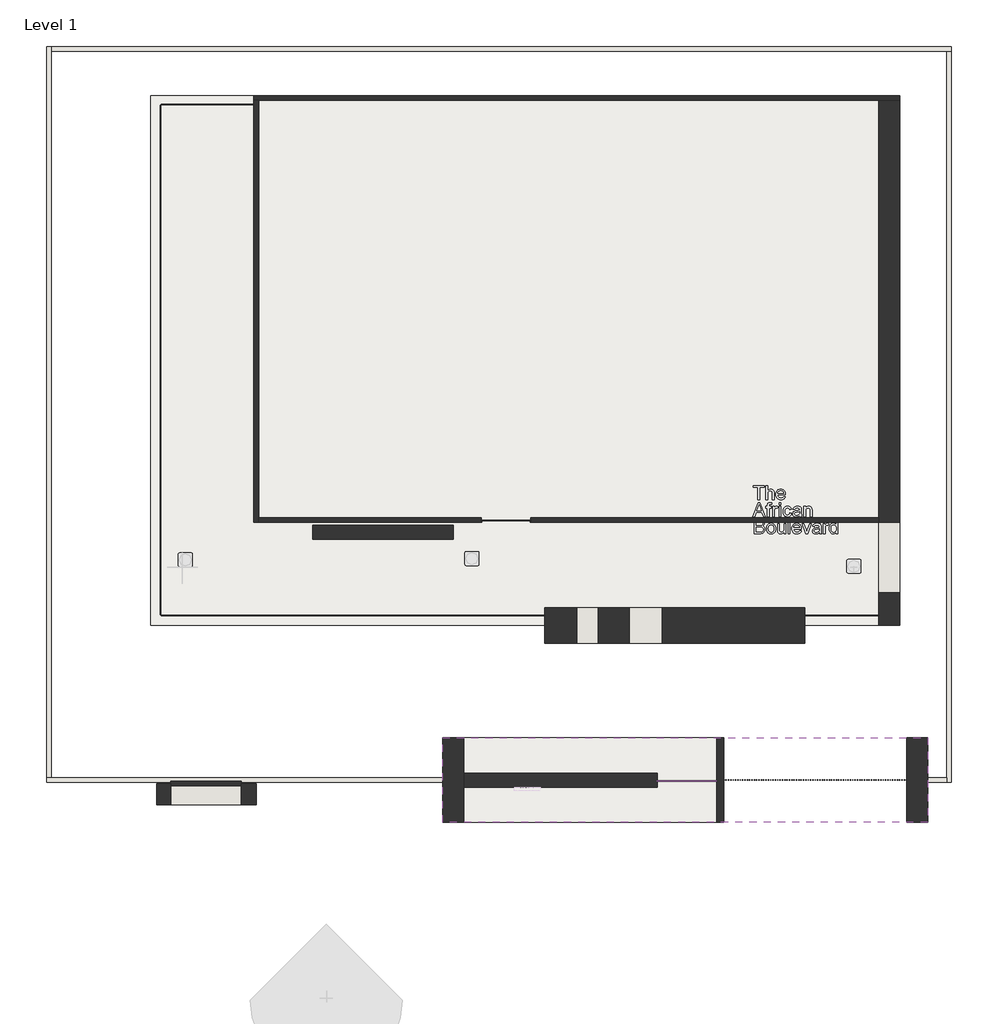
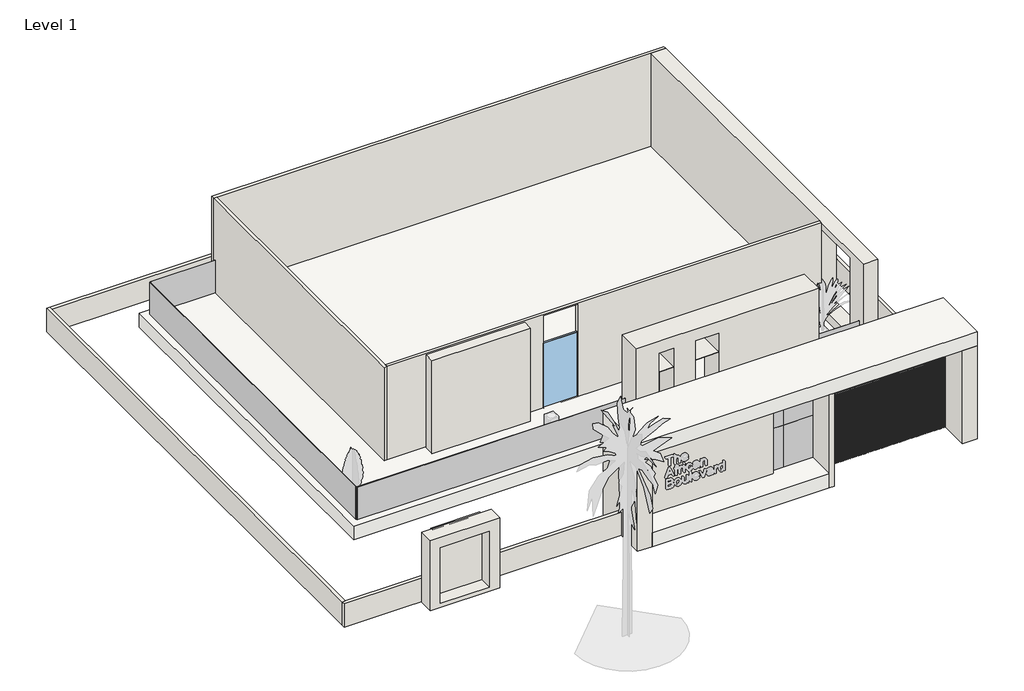
# One storey, part 1 of 3: 17 walls, 8 plates, 3 slabs, 1 railing, 1 window.
"""IFC4 building model written with IfcOpenShell, lengths in millimetres."""

from ifc_helpers import new_model, si_unit, frame, origin, origin_with_axes, place, context, project, spatial, polyline, outline, extrude, faceted_brep, transform, mapped, element, save
from components import system_panel_glazed_7ce5a3c2, system_panel_glazed_6867f845, system_panel_glazed_ba49168f, system_panel_glazed_c41ca4f4, system_panel_glazed_b21aad5f, system_panel_glazed_a143568c, system_panel_glazed_20dba380, system_panel_glazed_7cdb8ab2, window_2382273a

model = new_model("IFC4")

# Units and contexts
model_context = context("Model", 3, world=origin())
ifc_project = project(units=[si_unit("LENGTHUNIT", "METRE", prefix="MILLI")], contexts=[model_context])

# Site, building, storey
site = spatial("IfcSite", under=ifc_project)
building = spatial("IfcBuilding", under=site)
storey = spatial("IfcBuildingStorey", under=building, Name="Level 1", Elevation=0.0)

# Plates
placement = place(None, origin())
system_panel_glazed_shape = system_panel_glazed_7ce5a3c2(model_context)
element("IfcPlate", 1, ObjectType="System Panel : Glazed", at=placement, inside=storey, context=model_context, shape_type="MappedRepresentation", body=[
    mapped(system_panel_glazed_shape, transform((3844.4125281, -5000.7632813, 0.0), x_axis=(-1.0, 0.0, 0.0), y_axis=(0.0, -1.0, 0.0), z_axis=(0.0, 0.0, 1.0))),
])
system_panel_glazed_2_shape = system_panel_glazed_6867f845(model_context)
element("IfcPlate", 2, ObjectType="System Panel : Glazed", at=placement, inside=storey, context=model_context, shape_type="MappedRepresentation", body=[
    mapped(system_panel_glazed_2_shape, transform((-17339.1874719, -5000.7632813, 0.0), x_axis=(-1.0, 0.0, 0.0), y_axis=(0.0, -1.0, 0.0), z_axis=(0.0, 0.0, 1.0))),
])
system_panel_glazed_3_shape = system_panel_glazed_ba49168f(model_context)
element("IfcPlate", 3, ObjectType="System Panel : Glazed", at=placement, inside=storey, context=model_context, shape_type="MappedRepresentation", body=[
    mapped(system_panel_glazed_3_shape, transform((-25644.9874719, 6048.2367187, 0.0), x_axis=(0.0, 1.0, 0.0), y_axis=(-1.0, 0.0, 0.0), z_axis=(0.0, 0.0, 1.0))),
])
system_panel_glazed_4_shape = system_panel_glazed_c41ca4f4(model_context)
element("IfcPlate", 4, ObjectType="System Panel : Glazed", at=placement, inside=storey, context=model_context, shape_type="MappedRepresentation", body=[
    mapped(system_panel_glazed_4_shape, transform((-23638.3874719, 17097.2367187, 0.0), x_axis=(1.0, 0.0, 0.0), y_axis=(0.0, 1.0, 0.0), z_axis=(0.0, 0.0, 1.0))),
])
system_panel_glazed_5_shape = system_panel_glazed_b21aad5f(model_context)
element("IfcPlate", 5, ObjectType="System Panel : Glazed", at=placement, inside=storey, context=model_context, shape_type="MappedRepresentation", body=[
    mapped(system_panel_glazed_5_shape, transform((-2480.1874719, -12163.5632813, -914.4), x_axis=(-1.0, 0.0, 0.0), y_axis=(0.0, -1.0, 0.0), z_axis=(0.0, 0.0, 1.0))),
])
system_panel_glazed_6_shape = system_panel_glazed_a143568c(model_context)
element("IfcPlate", 6, ObjectType="System Panel : Glazed", at=placement, inside=storey, context=model_context, shape_type="MappedRepresentation", body=[
    mapped(system_panel_glazed_6_shape, transform((-2480.1874719, -12163.5632813, 2743.2), x_axis=(-1.0, 0.0, 0.0), y_axis=(0.0, -1.0, 0.0), z_axis=(0.0, 0.0, 1.0))),
])
system_panel_glazed_7_shape = system_panel_glazed_20dba380(model_context)
element("IfcPlate", 7, ObjectType="System Panel : Glazed", at=placement, inside=storey, context=model_context, shape_type="MappedRepresentation", body=[
    mapped(system_panel_glazed_7_shape, transform((-3775.5874719, -12163.5632813, -914.4), x_axis=(-1.0, 0.0, 0.0), y_axis=(0.0, -1.0, 0.0), z_axis=(0.0, 0.0, 1.0))),
])
system_panel_glazed_8_shape = system_panel_glazed_7cdb8ab2(model_context)
element("IfcPlate", 8, ObjectType="System Panel : Glazed", at=placement, inside=storey, context=model_context, shape_type="MappedRepresentation", body=[
    mapped(system_panel_glazed_8_shape, transform((-3775.5874719, -12163.5632813, 2743.2), x_axis=(-1.0, 0.0, 0.0), y_axis=(0.0, -1.0, 0.0), z_axis=(0.0, 0.0, 1.0))),
])

# Railing
element("IfcRailing", 9, ObjectType="Handrail - Rectangular", at=placement, inside=storey, context=model_context, shape_type="SweptSolid", body=[
    extrude(outline(polyline([(6663.8125281, -12138.1632813), (6663.8125281, -12188.9632813), (-1413.3874719, -12188.9632813), (-1413.3874719, -12138.1632813), (6663.8125281, -12138.1632813)])), frame((0.0, 0.0, 3606.8), z_axis=(0.0, 0.0, 1.0), x_axis=(1.0, 0.0, 0.0)), (0.0, 0.0, 1.0), 50.8),
    extrude(outline(polyline([(-1353.0624719, -12154.0382813), (-1353.0624719, -12173.0882813), (-1372.1124719, -12173.0882813), (-1372.1124719, -12154.0382813), (-1353.0624719, -12154.0382813)])), frame((0.0, 0.0, -914.4), z_axis=(0.0, 0.0, 1.0), x_axis=(1.0, 0.0, 0.0)), (0.0, 0.0, 1.0), 4521.2),
    extrude(outline(polyline([(-1251.4624719, -12154.0382813), (-1251.4624719, -12173.0882813), (-1270.5124719, -12173.0882813), (-1270.5124719, -12154.0382813), (-1251.4624719, -12154.0382813)])), frame((0.0, 0.0, -914.4), z_axis=(0.0, 0.0, 1.0), x_axis=(1.0, 0.0, 0.0)), (0.0, 0.0, 1.0), 4521.2),
    extrude(outline(polyline([(-1149.8624719, -12154.0382813), (-1149.8624719, -12173.0882813), (-1168.9124719, -12173.0882813), (-1168.9124719, -12154.0382813), (-1149.8624719, -12154.0382813)])), frame((0.0, 0.0, -914.4), z_axis=(0.0, 0.0, 1.0), x_axis=(1.0, 0.0, 0.0)), (0.0, 0.0, 1.0), 4521.2),
    extrude(outline(polyline([(-1048.2624719, -12154.0382813), (-1048.2624719, -12173.0882813), (-1067.3124719, -12173.0882813), (-1067.3124719, -12154.0382813), (-1048.2624719, -12154.0382813)])), frame((0.0, 0.0, -914.4), z_axis=(0.0, 0.0, 1.0), x_axis=(1.0, 0.0, 0.0)), (0.0, 0.0, 1.0), 4521.2),
    extrude(outline(polyline([(-946.6624719, -12154.0382813), (-946.6624719, -12173.0882813), (-965.7124719, -12173.0882813), (-965.7124719, -12154.0382813), (-946.6624719, -12154.0382813)])), frame((0.0, 0.0, -914.4), z_axis=(0.0, 0.0, 1.0), x_axis=(1.0, 0.0, 0.0)), (0.0, 0.0, 1.0), 4521.2),
    extrude(outline(polyline([(-845.0624719, -12154.0382813), (-845.0624719, -12173.0882813), (-864.1124719, -12173.0882813), (-864.1124719, -12154.0382813), (-845.0624719, -12154.0382813)])), frame((0.0, 0.0, -914.4), z_axis=(0.0, 0.0, 1.0), x_axis=(1.0, 0.0, 0.0)), (0.0, 0.0, 1.0), 4521.2),
    extrude(outline(polyline([(-743.4624719, -12154.0382813), (-743.4624719, -12173.0882813), (-762.5124719, -12173.0882813), (-762.5124719, -12154.0382813), (-743.4624719, -12154.0382813)])), frame((0.0, 0.0, -914.4), z_axis=(0.0, 0.0, 1.0), x_axis=(1.0, 0.0, 0.0)), (0.0, 0.0, 1.0), 4521.2),
    extrude(outline(polyline([(-641.8624719, -12154.0382813), (-641.8624719, -12173.0882813), (-660.9124719, -12173.0882813), (-660.9124719, -12154.0382813), (-641.8624719, -12154.0382813)])), frame((0.0, 0.0, -914.4), z_axis=(0.0, 0.0, 1.0), x_axis=(1.0, 0.0, 0.0)), (0.0, 0.0, 1.0), 4521.2),
    extrude(outline(polyline([(-540.2624719, -12154.0382813), (-540.2624719, -12173.0882813), (-559.3124719, -12173.0882813), (-559.3124719, -12154.0382813), (-540.2624719, -12154.0382813)])), frame((0.0, 0.0, -914.4), z_axis=(0.0, 0.0, 1.0), x_axis=(1.0, 0.0, 0.0)), (0.0, 0.0, 1.0), 4521.2),
    extrude(outline(polyline([(-438.6624719, -12154.0382813), (-438.6624719, -12173.0882813), (-457.7124719, -12173.0882813), (-457.7124719, -12154.0382813), (-438.6624719, -12154.0382813)])), frame((0.0, 0.0, -914.4), z_axis=(0.0, 0.0, 1.0), x_axis=(1.0, 0.0, 0.0)), (0.0, 0.0, 1.0), 4521.2),
    extrude(outline(polyline([(-337.0624719, -12154.0382813), (-337.0624719, -12173.0882813), (-356.1124719, -12173.0882813), (-356.1124719, -12154.0382813), (-337.0624719, -12154.0382813)])), frame((0.0, 0.0, -914.4), z_axis=(0.0, 0.0, 1.0), x_axis=(1.0, 0.0, 0.0)), (0.0, 0.0, 1.0), 4521.2),
    extrude(outline(polyline([(-235.4624719, -12154.0382813), (-235.4624719, -12173.0882813), (-254.5124719, -12173.0882813), (-254.5124719, -12154.0382813), (-235.4624719, -12154.0382813)])), frame((0.0, 0.0, -914.4), z_axis=(0.0, 0.0, 1.0), x_axis=(1.0, 0.0, 0.0)), (0.0, 0.0, 1.0), 4521.2),
    extrude(outline(polyline([(-133.8624719, -12154.0382813), (-133.8624719, -12173.0882813), (-152.9124719, -12173.0882813), (-152.9124719, -12154.0382813), (-133.8624719, -12154.0382813)])), frame((0.0, 0.0, -914.4), z_axis=(0.0, 0.0, 1.0), x_axis=(1.0, 0.0, 0.0)), (0.0, 0.0, 1.0), 4521.2),
    extrude(outline(polyline([(-32.2624719, -12154.0382813), (-32.2624719, -12173.0882813), (-51.3124719, -12173.0882813), (-51.3124719, -12154.0382813), (-32.2624719, -12154.0382813)])), frame((0.0, 0.0, -914.4), z_axis=(0.0, 0.0, 1.0), x_axis=(1.0, 0.0, 0.0)), (0.0, 0.0, 1.0), 4521.2),
    extrude(outline(polyline([(69.3375281, -12154.0382813), (69.3375281, -12173.0882813), (50.2875281, -12173.0882813), (50.2875281, -12154.0382813), (69.3375281, -12154.0382813)])), frame((0.0, 0.0, -914.4), z_axis=(0.0, 0.0, 1.0), x_axis=(1.0, 0.0, 0.0)), (0.0, 0.0, 1.0), 4521.2),
    extrude(outline(polyline([(170.9375281, -12154.0382813), (170.9375281, -12173.0882813), (151.8875281, -12173.0882813), (151.8875281, -12154.0382813), (170.9375281, -12154.0382813)])), frame((0.0, 0.0, -914.4), z_axis=(0.0, 0.0, 1.0), x_axis=(1.0, 0.0, 0.0)), (0.0, 0.0, 1.0), 4521.2),
    extrude(outline(polyline([(272.5375281, -12154.0382813), (272.5375281, -12173.0882813), (253.4875281, -12173.0882813), (253.4875281, -12154.0382813), (272.5375281, -12154.0382813)])), frame((0.0, 0.0, -914.4), z_axis=(0.0, 0.0, 1.0), x_axis=(1.0, 0.0, 0.0)), (0.0, 0.0, 1.0), 4521.2),
    extrude(outline(polyline([(374.1375281, -12154.0382813), (374.1375281, -12173.0882813), (355.0875281, -12173.0882813), (355.0875281, -12154.0382813), (374.1375281, -12154.0382813)])), frame((0.0, 0.0, -914.4), z_axis=(0.0, 0.0, 1.0), x_axis=(1.0, 0.0, 0.0)), (0.0, 0.0, 1.0), 4521.2),
    extrude(outline(polyline([(475.7375281, -12154.0382813), (475.7375281, -12173.0882813), (456.6875281, -12173.0882813), (456.6875281, -12154.0382813), (475.7375281, -12154.0382813)])), frame((0.0, 0.0, -914.4), z_axis=(0.0, 0.0, 1.0), x_axis=(1.0, 0.0, 0.0)), (0.0, 0.0, 1.0), 4521.2),
    extrude(outline(polyline([(577.3375281, -12154.0382813), (577.3375281, -12173.0882813), (558.2875281, -12173.0882813), (558.2875281, -12154.0382813), (577.3375281, -12154.0382813)])), frame((0.0, 0.0, -914.4), z_axis=(0.0, 0.0, 1.0), x_axis=(1.0, 0.0, 0.0)), (0.0, 0.0, 1.0), 4521.2),
    extrude(outline(polyline([(678.9375281, -12154.0382813), (678.9375281, -12173.0882813), (659.8875281, -12173.0882813), (659.8875281, -12154.0382813), (678.9375281, -12154.0382813)])), frame((0.0, 0.0, -914.4), z_axis=(0.0, 0.0, 1.0), x_axis=(1.0, 0.0, 0.0)), (0.0, 0.0, 1.0), 4521.2),
    extrude(outline(polyline([(780.5375281, -12154.0382813), (780.5375281, -12173.0882813), (761.4875281, -12173.0882813), (761.4875281, -12154.0382813), (780.5375281, -12154.0382813)])), frame((0.0, 0.0, -914.4), z_axis=(0.0, 0.0, 1.0), x_axis=(1.0, 0.0, 0.0)), (0.0, 0.0, 1.0), 4521.2),
    extrude(outline(polyline([(882.1375281, -12154.0382813), (882.1375281, -12173.0882813), (863.0875281, -12173.0882813), (863.0875281, -12154.0382813), (882.1375281, -12154.0382813)])), frame((0.0, 0.0, -914.4), z_axis=(0.0, 0.0, 1.0), x_axis=(1.0, 0.0, 0.0)), (0.0, 0.0, 1.0), 4521.2),
    extrude(outline(polyline([(983.7375281, -12154.0382813), (983.7375281, -12173.0882813), (964.6875281, -12173.0882813), (964.6875281, -12154.0382813), (983.7375281, -12154.0382813)])), frame((0.0, 0.0, -914.4), z_axis=(0.0, 0.0, 1.0), x_axis=(1.0, 0.0, 0.0)), (0.0, 0.0, 1.0), 4521.2),
    extrude(outline(polyline([(1085.3375281, -12154.0382813), (1085.3375281, -12173.0882813), (1066.2875281, -12173.0882813), (1066.2875281, -12154.0382813), (1085.3375281, -12154.0382813)])), frame((0.0, 0.0, -914.4), z_axis=(0.0, 0.0, 1.0), x_axis=(1.0, 0.0, 0.0)), (0.0, 0.0, 1.0), 4521.2),
    extrude(outline(polyline([(1186.9375281, -12154.0382813), (1186.9375281, -12173.0882813), (1167.8875281, -12173.0882813), (1167.8875281, -12154.0382813), (1186.9375281, -12154.0382813)])), frame((0.0, 0.0, -914.4), z_axis=(0.0, 0.0, 1.0), x_axis=(1.0, 0.0, 0.0)), (0.0, 0.0, 1.0), 4521.2),
    extrude(outline(polyline([(1288.5375281, -12154.0382813), (1288.5375281, -12173.0882813), (1269.4875281, -12173.0882813), (1269.4875281, -12154.0382813), (1288.5375281, -12154.0382813)])), frame((0.0, 0.0, -914.4), z_axis=(0.0, 0.0, 1.0), x_axis=(1.0, 0.0, 0.0)), (0.0, 0.0, 1.0), 4521.2),
    extrude(outline(polyline([(1390.1375281, -12154.0382813), (1390.1375281, -12173.0882813), (1371.0875281, -12173.0882813), (1371.0875281, -12154.0382813), (1390.1375281, -12154.0382813)])), frame((0.0, 0.0, -914.4), z_axis=(0.0, 0.0, 1.0), x_axis=(1.0, 0.0, 0.0)), (0.0, 0.0, 1.0), 4521.2),
    extrude(outline(polyline([(1491.7375281, -12154.0382813), (1491.7375281, -12173.0882813), (1472.6875281, -12173.0882813), (1472.6875281, -12154.0382813), (1491.7375281, -12154.0382813)])), frame((0.0, 0.0, -914.4), z_axis=(0.0, 0.0, 1.0), x_axis=(1.0, 0.0, 0.0)), (0.0, 0.0, 1.0), 4521.2),
    extrude(outline(polyline([(1593.3375281, -12154.0382813), (1593.3375281, -12173.0882813), (1574.2875281, -12173.0882813), (1574.2875281, -12154.0382813), (1593.3375281, -12154.0382813)])), frame((0.0, 0.0, -914.4), z_axis=(0.0, 0.0, 1.0), x_axis=(1.0, 0.0, 0.0)), (0.0, 0.0, 1.0), 4521.2),
    extrude(outline(polyline([(1694.9375281, -12154.0382813), (1694.9375281, -12173.0882813), (1675.8875281, -12173.0882813), (1675.8875281, -12154.0382813), (1694.9375281, -12154.0382813)])), frame((0.0, 0.0, -914.4), z_axis=(0.0, 0.0, 1.0), x_axis=(1.0, 0.0, 0.0)), (0.0, 0.0, 1.0), 4521.2),
    extrude(outline(polyline([(1796.5375281, -12154.0382813), (1796.5375281, -12173.0882813), (1777.4875281, -12173.0882813), (1777.4875281, -12154.0382813), (1796.5375281, -12154.0382813)])), frame((0.0, 0.0, -914.4), z_axis=(0.0, 0.0, 1.0), x_axis=(1.0, 0.0, 0.0)), (0.0, 0.0, 1.0), 4521.2),
    extrude(outline(polyline([(1898.1375281, -12154.0382813), (1898.1375281, -12173.0882813), (1879.0875281, -12173.0882813), (1879.0875281, -12154.0382813), (1898.1375281, -12154.0382813)])), frame((0.0, 0.0, -914.4), z_axis=(0.0, 0.0, 1.0), x_axis=(1.0, 0.0, 0.0)), (0.0, 0.0, 1.0), 4521.2),
    extrude(outline(polyline([(1999.7375281, -12154.0382813), (1999.7375281, -12173.0882813), (1980.6875281, -12173.0882813), (1980.6875281, -12154.0382813), (1999.7375281, -12154.0382813)])), frame((0.0, 0.0, -914.4), z_axis=(0.0, 0.0, 1.0), x_axis=(1.0, 0.0, 0.0)), (0.0, 0.0, 1.0), 4521.2),
    extrude(outline(polyline([(2101.3375281, -12154.0382813), (2101.3375281, -12173.0882813), (2082.2875281, -12173.0882813), (2082.2875281, -12154.0382813), (2101.3375281, -12154.0382813)])), frame((0.0, 0.0, -914.4), z_axis=(0.0, 0.0, 1.0), x_axis=(1.0, 0.0, 0.0)), (0.0, 0.0, 1.0), 4521.2),
    extrude(outline(polyline([(2202.9375281, -12154.0382813), (2202.9375281, -12173.0882813), (2183.8875281, -12173.0882813), (2183.8875281, -12154.0382813), (2202.9375281, -12154.0382813)])), frame((0.0, 0.0, -914.4), z_axis=(0.0, 0.0, 1.0), x_axis=(1.0, 0.0, 0.0)), (0.0, 0.0, 1.0), 4521.2),
    extrude(outline(polyline([(2304.5375281, -12154.0382813), (2304.5375281, -12173.0882813), (2285.4875281, -12173.0882813), (2285.4875281, -12154.0382813), (2304.5375281, -12154.0382813)])), frame((0.0, 0.0, -914.4), z_axis=(0.0, 0.0, 1.0), x_axis=(1.0, 0.0, 0.0)), (0.0, 0.0, 1.0), 4521.2),
    extrude(outline(polyline([(2406.1375281, -12154.0382813), (2406.1375281, -12173.0882813), (2387.0875281, -12173.0882813), (2387.0875281, -12154.0382813), (2406.1375281, -12154.0382813)])), frame((0.0, 0.0, -914.4), z_axis=(0.0, 0.0, 1.0), x_axis=(1.0, 0.0, 0.0)), (0.0, 0.0, 1.0), 4521.2),
    extrude(outline(polyline([(2507.7375281, -12154.0382813), (2507.7375281, -12173.0882813), (2488.6875281, -12173.0882813), (2488.6875281, -12154.0382813), (2507.7375281, -12154.0382813)])), frame((0.0, 0.0, -914.4), z_axis=(0.0, 0.0, 1.0), x_axis=(1.0, 0.0, 0.0)), (0.0, 0.0, 1.0), 4521.2),
    extrude(outline(polyline([(2609.3375281, -12154.0382813), (2609.3375281, -12173.0882813), (2590.2875281, -12173.0882813), (2590.2875281, -12154.0382813), (2609.3375281, -12154.0382813)])), frame((0.0, 0.0, -914.4), z_axis=(0.0, 0.0, 1.0), x_axis=(1.0, 0.0, 0.0)), (0.0, 0.0, 1.0), 4521.2),
    extrude(outline(polyline([(2710.9375281, -12154.0382813), (2710.9375281, -12173.0882813), (2691.8875281, -12173.0882813), (2691.8875281, -12154.0382813), (2710.9375281, -12154.0382813)])), frame((0.0, 0.0, -914.4), z_axis=(0.0, 0.0, 1.0), x_axis=(1.0, 0.0, 0.0)), (0.0, 0.0, 1.0), 4521.2),
    extrude(outline(polyline([(2812.5375281, -12154.0382813), (2812.5375281, -12173.0882813), (2793.4875281, -12173.0882813), (2793.4875281, -12154.0382813), (2812.5375281, -12154.0382813)])), frame((0.0, 0.0, -914.4), z_axis=(0.0, 0.0, 1.0), x_axis=(1.0, 0.0, 0.0)), (0.0, 0.0, 1.0), 4521.2),
    extrude(outline(polyline([(2914.1375281, -12154.0382813), (2914.1375281, -12173.0882813), (2895.0875281, -12173.0882813), (2895.0875281, -12154.0382813), (2914.1375281, -12154.0382813)])), frame((0.0, 0.0, -914.4), z_axis=(0.0, 0.0, 1.0), x_axis=(1.0, 0.0, 0.0)), (0.0, 0.0, 1.0), 4521.2),
    extrude(outline(polyline([(3015.7375281, -12154.0382813), (3015.7375281, -12173.0882813), (2996.6875281, -12173.0882813), (2996.6875281, -12154.0382813), (3015.7375281, -12154.0382813)])), frame((0.0, 0.0, -914.4), z_axis=(0.0, 0.0, 1.0), x_axis=(1.0, 0.0, 0.0)), (0.0, 0.0, 1.0), 4521.2),
    extrude(outline(polyline([(3117.3375281, -12154.0382813), (3117.3375281, -12173.0882813), (3098.2875281, -12173.0882813), (3098.2875281, -12154.0382813), (3117.3375281, -12154.0382813)])), frame((0.0, 0.0, -914.4), z_axis=(0.0, 0.0, 1.0), x_axis=(1.0, 0.0, 0.0)), (0.0, 0.0, 1.0), 4521.2),
    extrude(outline(polyline([(3218.9375281, -12154.0382813), (3218.9375281, -12173.0882813), (3199.8875281, -12173.0882813), (3199.8875281, -12154.0382813), (3218.9375281, -12154.0382813)])), frame((0.0, 0.0, -914.4), z_axis=(0.0, 0.0, 1.0), x_axis=(1.0, 0.0, 0.0)), (0.0, 0.0, 1.0), 4521.2),
    extrude(outline(polyline([(3320.5375281, -12154.0382813), (3320.5375281, -12173.0882813), (3301.4875281, -12173.0882813), (3301.4875281, -12154.0382813), (3320.5375281, -12154.0382813)])), frame((0.0, 0.0, -914.4), z_axis=(0.0, 0.0, 1.0), x_axis=(1.0, 0.0, 0.0)), (0.0, 0.0, 1.0), 4521.2),
    extrude(outline(polyline([(3422.1375281, -12154.0382813), (3422.1375281, -12173.0882813), (3403.0875281, -12173.0882813), (3403.0875281, -12154.0382813), (3422.1375281, -12154.0382813)])), frame((0.0, 0.0, -914.4), z_axis=(0.0, 0.0, 1.0), x_axis=(1.0, 0.0, 0.0)), (0.0, 0.0, 1.0), 4521.2),
    extrude(outline(polyline([(3523.7375281, -12154.0382813), (3523.7375281, -12173.0882813), (3504.6875281, -12173.0882813), (3504.6875281, -12154.0382813), (3523.7375281, -12154.0382813)])), frame((0.0, 0.0, -914.4), z_axis=(0.0, 0.0, 1.0), x_axis=(1.0, 0.0, 0.0)), (0.0, 0.0, 1.0), 4521.2),
    extrude(outline(polyline([(3625.3375281, -12154.0382813), (3625.3375281, -12173.0882813), (3606.2875281, -12173.0882813), (3606.2875281, -12154.0382813), (3625.3375281, -12154.0382813)])), frame((0.0, 0.0, -914.4), z_axis=(0.0, 0.0, 1.0), x_axis=(1.0, 0.0, 0.0)), (0.0, 0.0, 1.0), 4521.2),
    extrude(outline(polyline([(3726.9375281, -12154.0382813), (3726.9375281, -12173.0882813), (3707.8875281, -12173.0882813), (3707.8875281, -12154.0382813), (3726.9375281, -12154.0382813)])), frame((0.0, 0.0, -914.4), z_axis=(0.0, 0.0, 1.0), x_axis=(1.0, 0.0, 0.0)), (0.0, 0.0, 1.0), 4521.2),
    extrude(outline(polyline([(3828.5375281, -12154.0382813), (3828.5375281, -12173.0882813), (3809.4875281, -12173.0882813), (3809.4875281, -12154.0382813), (3828.5375281, -12154.0382813)])), frame((0.0, 0.0, -914.4), z_axis=(0.0, 0.0, 1.0), x_axis=(1.0, 0.0, 0.0)), (0.0, 0.0, 1.0), 4521.2),
    extrude(outline(polyline([(3930.1375281, -12154.0382813), (3930.1375281, -12173.0882813), (3911.0875281, -12173.0882813), (3911.0875281, -12154.0382813), (3930.1375281, -12154.0382813)])), frame((0.0, 0.0, -914.4), z_axis=(0.0, 0.0, 1.0), x_axis=(1.0, 0.0, 0.0)), (0.0, 0.0, 1.0), 4521.2),
    extrude(outline(polyline([(4031.7375281, -12154.0382813), (4031.7375281, -12173.0882813), (4012.6875281, -12173.0882813), (4012.6875281, -12154.0382813), (4031.7375281, -12154.0382813)])), frame((0.0, 0.0, -914.4), z_axis=(0.0, 0.0, 1.0), x_axis=(1.0, 0.0, 0.0)), (0.0, 0.0, 1.0), 4521.2),
    extrude(outline(polyline([(4133.3375281, -12154.0382813), (4133.3375281, -12173.0882813), (4114.2875281, -12173.0882813), (4114.2875281, -12154.0382813), (4133.3375281, -12154.0382813)])), frame((0.0, 0.0, -914.4), z_axis=(0.0, 0.0, 1.0), x_axis=(1.0, 0.0, 0.0)), (0.0, 0.0, 1.0), 4521.2),
    extrude(outline(polyline([(4234.9375281, -12154.0382813), (4234.9375281, -12173.0882813), (4215.8875281, -12173.0882813), (4215.8875281, -12154.0382813), (4234.9375281, -12154.0382813)])), frame((0.0, 0.0, -914.4), z_axis=(0.0, 0.0, 1.0), x_axis=(1.0, 0.0, 0.0)), (0.0, 0.0, 1.0), 4521.2),
    extrude(outline(polyline([(4336.5375281, -12154.0382813), (4336.5375281, -12173.0882813), (4317.4875281, -12173.0882813), (4317.4875281, -12154.0382813), (4336.5375281, -12154.0382813)])), frame((0.0, 0.0, -914.4), z_axis=(0.0, 0.0, 1.0), x_axis=(1.0, 0.0, 0.0)), (0.0, 0.0, 1.0), 4521.2),
    extrude(outline(polyline([(4438.1375281, -12154.0382813), (4438.1375281, -12173.0882813), (4419.0875281, -12173.0882813), (4419.0875281, -12154.0382813), (4438.1375281, -12154.0382813)])), frame((0.0, 0.0, -914.4), z_axis=(0.0, 0.0, 1.0), x_axis=(1.0, 0.0, 0.0)), (0.0, 0.0, 1.0), 4521.2),
    extrude(outline(polyline([(4539.7375281, -12154.0382813), (4539.7375281, -12173.0882813), (4520.6875281, -12173.0882813), (4520.6875281, -12154.0382813), (4539.7375281, -12154.0382813)])), frame((0.0, 0.0, -914.4), z_axis=(0.0, 0.0, 1.0), x_axis=(1.0, 0.0, 0.0)), (0.0, 0.0, 1.0), 4521.2),
    extrude(outline(polyline([(4641.3375281, -12154.0382813), (4641.3375281, -12173.0882813), (4622.2875281, -12173.0882813), (4622.2875281, -12154.0382813), (4641.3375281, -12154.0382813)])), frame((0.0, 0.0, -914.4), z_axis=(0.0, 0.0, 1.0), x_axis=(1.0, 0.0, 0.0)), (0.0, 0.0, 1.0), 4521.2),
    extrude(outline(polyline([(4742.9375281, -12154.0382813), (4742.9375281, -12173.0882813), (4723.8875281, -12173.0882813), (4723.8875281, -12154.0382813), (4742.9375281, -12154.0382813)])), frame((0.0, 0.0, -914.4), z_axis=(0.0, 0.0, 1.0), x_axis=(1.0, 0.0, 0.0)), (0.0, 0.0, 1.0), 4521.2),
    extrude(outline(polyline([(4844.5375281, -12154.0382813), (4844.5375281, -12173.0882813), (4825.4875281, -12173.0882813), (4825.4875281, -12154.0382813), (4844.5375281, -12154.0382813)])), frame((0.0, 0.0, -914.4), z_axis=(0.0, 0.0, 1.0), x_axis=(1.0, 0.0, 0.0)), (0.0, 0.0, 1.0), 4521.2),
    extrude(outline(polyline([(4946.1375281, -12154.0382813), (4946.1375281, -12173.0882813), (4927.0875281, -12173.0882813), (4927.0875281, -12154.0382813), (4946.1375281, -12154.0382813)])), frame((0.0, 0.0, -914.4), z_axis=(0.0, 0.0, 1.0), x_axis=(1.0, 0.0, 0.0)), (0.0, 0.0, 1.0), 4521.2),
    extrude(outline(polyline([(5047.7375281, -12154.0382813), (5047.7375281, -12173.0882813), (5028.6875281, -12173.0882813), (5028.6875281, -12154.0382813), (5047.7375281, -12154.0382813)])), frame((0.0, 0.0, -914.4), z_axis=(0.0, 0.0, 1.0), x_axis=(1.0, 0.0, 0.0)), (0.0, 0.0, 1.0), 4521.2),
    extrude(outline(polyline([(5149.3375281, -12154.0382813), (5149.3375281, -12173.0882813), (5130.2875281, -12173.0882813), (5130.2875281, -12154.0382813), (5149.3375281, -12154.0382813)])), frame((0.0, 0.0, -914.4), z_axis=(0.0, 0.0, 1.0), x_axis=(1.0, 0.0, 0.0)), (0.0, 0.0, 1.0), 4521.2),
    extrude(outline(polyline([(5250.9375281, -12154.0382813), (5250.9375281, -12173.0882813), (5231.8875281, -12173.0882813), (5231.8875281, -12154.0382813), (5250.9375281, -12154.0382813)])), frame((0.0, 0.0, -914.4), z_axis=(0.0, 0.0, 1.0), x_axis=(1.0, 0.0, 0.0)), (0.0, 0.0, 1.0), 4521.2),
    extrude(outline(polyline([(5352.5375281, -12154.0382813), (5352.5375281, -12173.0882813), (5333.4875281, -12173.0882813), (5333.4875281, -12154.0382813), (5352.5375281, -12154.0382813)])), frame((0.0, 0.0, -914.4), z_axis=(0.0, 0.0, 1.0), x_axis=(1.0, 0.0, 0.0)), (0.0, 0.0, 1.0), 4521.2),
    extrude(outline(polyline([(5454.1375281, -12154.0382813), (5454.1375281, -12173.0882813), (5435.0875281, -12173.0882813), (5435.0875281, -12154.0382813), (5454.1375281, -12154.0382813)])), frame((0.0, 0.0, -914.4), z_axis=(0.0, 0.0, 1.0), x_axis=(1.0, 0.0, 0.0)), (0.0, 0.0, 1.0), 4521.2),
    extrude(outline(polyline([(5555.7375281, -12154.0382813), (5555.7375281, -12173.0882813), (5536.6875281, -12173.0882813), (5536.6875281, -12154.0382813), (5555.7375281, -12154.0382813)])), frame((0.0, 0.0, -914.4), z_axis=(0.0, 0.0, 1.0), x_axis=(1.0, 0.0, 0.0)), (0.0, 0.0, 1.0), 4521.2),
    extrude(outline(polyline([(5657.3375281, -12154.0382813), (5657.3375281, -12173.0882813), (5638.2875281, -12173.0882813), (5638.2875281, -12154.0382813), (5657.3375281, -12154.0382813)])), frame((0.0, 0.0, -914.4), z_axis=(0.0, 0.0, 1.0), x_axis=(1.0, 0.0, 0.0)), (0.0, 0.0, 1.0), 4521.2),
    extrude(outline(polyline([(5758.9375281, -12154.0382813), (5758.9375281, -12173.0882813), (5739.8875281, -12173.0882813), (5739.8875281, -12154.0382813), (5758.9375281, -12154.0382813)])), frame((0.0, 0.0, -914.4), z_axis=(0.0, 0.0, 1.0), x_axis=(1.0, 0.0, 0.0)), (0.0, 0.0, 1.0), 4521.2),
    extrude(outline(polyline([(5860.5375281, -12154.0382813), (5860.5375281, -12173.0882813), (5841.4875281, -12173.0882813), (5841.4875281, -12154.0382813), (5860.5375281, -12154.0382813)])), frame((0.0, 0.0, -914.4), z_axis=(0.0, 0.0, 1.0), x_axis=(1.0, 0.0, 0.0)), (0.0, 0.0, 1.0), 4521.2),
    extrude(outline(polyline([(5962.1375281, -12154.0382813), (5962.1375281, -12173.0882813), (5943.0875281, -12173.0882813), (5943.0875281, -12154.0382813), (5962.1375281, -12154.0382813)])), frame((0.0, 0.0, -914.4), z_axis=(0.0, 0.0, 1.0), x_axis=(1.0, 0.0, 0.0)), (0.0, 0.0, 1.0), 4521.2),
    extrude(outline(polyline([(6063.7375281, -12154.0382813), (6063.7375281, -12173.0882813), (6044.6875281, -12173.0882813), (6044.6875281, -12154.0382813), (6063.7375281, -12154.0382813)])), frame((0.0, 0.0, -914.4), z_axis=(0.0, 0.0, 1.0), x_axis=(1.0, 0.0, 0.0)), (0.0, 0.0, 1.0), 4521.2),
    extrude(outline(polyline([(6165.3375281, -12154.0382813), (6165.3375281, -12173.0882813), (6146.2875281, -12173.0882813), (6146.2875281, -12154.0382813), (6165.3375281, -12154.0382813)])), frame((0.0, 0.0, -914.4), z_axis=(0.0, 0.0, 1.0), x_axis=(1.0, 0.0, 0.0)), (0.0, 0.0, 1.0), 4521.2),
    extrude(outline(polyline([(6266.9375281, -12154.0382813), (6266.9375281, -12173.0882813), (6247.8875281, -12173.0882813), (6247.8875281, -12154.0382813), (6266.9375281, -12154.0382813)])), frame((0.0, 0.0, -914.4), z_axis=(0.0, 0.0, 1.0), x_axis=(1.0, 0.0, 0.0)), (0.0, 0.0, 1.0), 4521.2),
    extrude(outline(polyline([(6368.5375281, -12154.0382813), (6368.5375281, -12173.0882813), (6349.4875281, -12173.0882813), (6349.4875281, -12154.0382813), (6368.5375281, -12154.0382813)])), frame((0.0, 0.0, -914.4), z_axis=(0.0, 0.0, 1.0), x_axis=(1.0, 0.0, 0.0)), (0.0, 0.0, 1.0), 4521.2),
    extrude(outline(polyline([(6470.1375281, -12154.0382813), (6470.1375281, -12173.0882813), (6451.0875281, -12173.0882813), (6451.0875281, -12154.0382813), (6470.1375281, -12154.0382813)])), frame((0.0, 0.0, -914.4), z_axis=(0.0, 0.0, 1.0), x_axis=(1.0, 0.0, 0.0)), (0.0, 0.0, 1.0), 4521.2),
    extrude(outline(polyline([(6571.7375281, -12154.0382813), (6571.7375281, -12173.0882813), (6552.6875281, -12173.0882813), (6552.6875281, -12154.0382813), (6571.7375281, -12154.0382813)])), frame((0.0, 0.0, -914.4), z_axis=(0.0, 0.0, 1.0), x_axis=(1.0, 0.0, 0.0)), (0.0, 0.0, 1.0), 4521.2),
    extrude(outline(polyline([(-1394.3374719, -12154.0382813), (-1394.3374719, -12173.0882813), (-1413.3874719, -12173.0882813), (-1413.3874719, -12154.0382813), (-1394.3374719, -12154.0382813)])), frame((0.0, 0.0, -914.4), z_axis=(0.0, 0.0, 1.0), x_axis=(1.0, 0.0, 0.0)), (0.0, 0.0, 1.0), 4521.2),
    extrude(outline(polyline([(6663.8125281, -12154.0382813), (6663.8125281, -12173.0882813), (6644.7625281, -12173.0882813), (6644.7625281, -12154.0382813), (6663.8125281, -12154.0382813)])), frame((0.0, 0.0, -914.4), z_axis=(0.0, 0.0, 1.0), x_axis=(1.0, 0.0, 0.0)), (0.0, 0.0, 1.0), 4521.2),
])

# Slabs
element("IfcSlab", 10, ObjectType="Generic - 3'", at=placement, inside=storey, context=model_context, shape_type="SweptSolid", body=[
    extrude(outline(polyline([(-26102.1874719, -5457.9632813), (-26102.1874719, 17503.6367187), (6359.0125281, 17503.6367187), (6359.0125281, -5457.9632813), (-26102.1874719, -5457.9632813)])), frame((0.0, 0.0, -914.4), z_axis=(0.0, 0.0, 1.0), x_axis=(1.0, 0.0, 0.0)), (0.0, 0.0, 1.0), 914.4),
])
element("IfcSlab", 11, ObjectType="Generic - 3'", at=placement, inside=storey, context=model_context, shape_type="SweptSolid", body=[
    extrude(outline(polyline([(-1565.7874719, -10334.7632813), (-1565.7874719, -13992.3632813), (-12538.5874719, -13992.3632813), (-12538.5874719, -10334.7632813), (-1565.7874719, -10334.7632813)])), frame((0.0, 0.0, -914.4), z_axis=(0.0, 0.0, 1.0), x_axis=(1.0, 0.0, 0.0)), (0.0, 0.0, 1.0), 914.4),
])
element("IfcSlab", 12, ObjectType="Generic - 3'", at=placement, inside=storey, context=model_context, shape_type="SweptSolid", body=[
    extrude(outline(polyline([(7578.2125281, -10334.7632813), (7578.2125281, -13992.3632813), (-13452.9874719, -13992.3632813), (-13452.9874719, -10334.7632813), (7578.2125281, -10334.7632813)])), frame((0.0, 0.0, 5181.6), z_axis=(0.0, 0.0, 1.0), x_axis=(1.0, 0.0, 0.0)), (0.0, 0.0, 1.0), 914.4),
])

# Walls
element("IfcWall", 13, ObjectType="Generic - 12\" 2", at=placement, inside=storey, context=model_context, shape_type="SweptSolid", body=[
    extrude(outline(polyline([(-1565.7874719, -13992.3632813), (-1565.7874719, -10334.7632813), (-1260.9874719, -10334.7632813), (-1260.9874719, -13992.3632813), (-1565.7874719, -13992.3632813)])), frame((0.0, 0.0, -914.4), z_axis=(0.0, 0.0, 1.0), x_axis=(1.0, 0.0, 0.0)), (0.0, 0.0, 1.0), 6096.0),
])
element("IfcWall", 14, ObjectType="Generic - 3'", at=placement, inside=storey, context=model_context, shape_type="Brep", body=[
    faceted_brep([(5444.6125281, 17300.4367187, 0.0), (5444.6125281, -784.3632813, 0.0), (5444.6125281, -987.5632813, 0.0), (5444.6125281, -5457.9632813, 0.0), (5444.6125281, -5457.9632813, 6096.0), (5444.6125281, -987.5632813, 6096.0), (5444.6125281, -784.3632813, 6096.0), (5444.6125281, 17300.4367187, 6096.0), (5444.6125281, -4035.5632813, 5648.487938), (5444.6125281, -4035.5632813, 619.287938), (5444.6125281, -987.5632813, 619.287938), (5444.6125281, -987.5632813, 5648.487938), (6359.0125281, 17300.4367187, 0.0), (6359.0125281, 17300.4367187, 6096.0), (6359.0125281, -5457.9632813, 6096.0), (6359.0125281, -5457.9632813, 0.0), (6359.0125281, -4035.5632813, 5648.487938), (6359.0125281, -987.5632813, 5648.487938), (6359.0125281, -987.5632813, 619.287938), (6359.0125281, -4035.5632813, 619.287938)], [[[0, 1, 2, 3, 4, 5, 6, 7], [8, 9, 10, 11]], [[12, 13, 14, 15], [16, 17, 18, 19]], [[0, 7, 13, 12]], [[3, 2, 1, 0, 12, 15]], [[4, 3, 15, 14]], [[7, 6, 5, 4, 14, 13]], [[9, 8, 16, 19]], [[10, 9, 19, 18]], [[8, 11, 17, 16]], [[11, 10, 18, 17]]]),
])
element("IfcWall", 15, ObjectType="Generic - 3'", at=placement, inside=storey, context=model_context, shape_type="Brep", body=[
    faceted_brep([(-13452.9874719, -10334.7632813, -914.4), (-13452.9874719, -12061.9632813, -914.4), (-13452.9874719, -12265.1632813, -914.4), (-13452.9874719, -13992.3632813, -914.4), (-13452.9874719, -13992.3632813, 5181.6), (-13452.9874719, -10334.7632813, 5181.6), (-12538.5874719, -10334.7632813, -914.4), (-12538.5874719, -10334.7632813, 5181.6), (-12538.5874719, -11858.7632813, 5181.6), (-12538.5874719, -12468.3632813, 5181.6), (-12538.5874719, -13992.3632813, 5181.6), (-12538.5874719, -13992.3632813, -914.4), (-12538.5874719, -12468.3632813, -914.4), (-12538.5874719, -11858.7632813, -914.4)], [[[0, 1, 2, 3, 4, 5]], [[6, 7, 8, 9, 10, 11, 12, 13]], [[3, 2, 1, 0, 6, 13, 12, 11]], [[4, 3, 11, 10]], [[5, 4, 10, 9, 8, 7]], [[0, 5, 7, 6]]]),
])
element("IfcWall", 16, ObjectType="Generic - 3'", at=placement, inside=storey, context=model_context, shape_type="Brep", body=[
    faceted_brep([(6663.8125281, -10334.7632813, -914.4), (6663.8125281, -13992.3632813, -914.4), (6663.8125281, -13992.3632813, 5181.6), (6663.8125281, -10334.7632813, 5181.6), (7578.2125281, -10334.7632813, -914.4), (7578.2125281, -10334.7632813, 5181.6), (7578.2125281, -13992.3632813, 5181.6), (7578.2125281, -13992.3632813, -914.4), (7578.2125281, -12265.1632813, -914.4), (7578.2125281, -12061.9632813, -914.4)], [[[0, 1, 2, 3]], [[4, 5, 6, 7, 8, 9]], [[1, 0, 4, 9, 8, 7]], [[2, 1, 7, 6]], [[3, 2, 6, 5]], [[0, 3, 5, 4]]]),
])
element("IfcWall", 17, ObjectType="Generic - 3'", at=placement, inside=storey, context=model_context, shape_type="SweptSolid", body=[
    extrude(outline(polyline([(-914.4, -25838.6624719), (-914.4, -21530.1874719), (3657.6, -21530.1874719), (3657.6, -25838.6624719), (-914.4, -25838.6624719)]), holes=[polyline([(2997.2, -22181.0624719), (-660.4, -22181.0624719), (-660.4, -25229.0624719), (2997.2, -25229.0624719), (2997.2, -22181.0624719)])]), frame((0.0, -13230.3632813, 0.0), z_axis=(0.0, 1.0, 0.0), x_axis=(0.0, 0.0, 1.0)), (0.0, 0.0, 1.0), 914.4),
])
element("IfcWall", 18, ObjectType="Generic - 3' gray", at=placement, inside=storey, context=model_context, shape_type="SweptSolid", body=[
    extrude(outline(polyline([(0.0, 2244.2125281), (6096.0, 2244.2125281), (6096.0, -9033.3874719), (0.0, -9033.3874719), (0.0, 2244.2125281)]), holes=[polyline([(5315.3308744, -6716.0306948), (4096.1308744, -6716.0306948), (4096.1308744, -7630.4306948), (5315.3308744, -7630.4306948), (5315.3308744, -6716.0306948)]), polyline([(286.1308744, -7630.4306948), (4070.7308744, -7630.4306948), (4070.7308744, -6716.0306948), (286.1308744, -6716.0306948), (286.1308744, -7630.4306948)]), polyline([(5315.3308744, -3924.8577662), (4096.1308744, -3924.8577662), (4096.1308744, -5371.4183212), (5315.3308744, -5371.4183212), (5315.3308744, -3924.8577662)]), polyline([(286.1308744, -5371.4183212), (4070.7308744, -5371.4183212), (4070.7308744, -3924.8577662), (286.1308744, -3924.8577662), (286.1308744, -5371.4183212)])]), frame((0.0, -6219.9632813, 0.0), z_axis=(0.0, 1.0, 0.0), x_axis=(0.0, 0.0, 1.0)), (0.0, 0.0, 1.0), 1524.0),
])
element("IfcWall", 19, ObjectType="Generic - 8\"", at=placement, inside=storey, context=model_context, shape_type="Brep", body=[
    faceted_brep([(-21631.7874719, 17300.4367187, 0.0), (-21428.5874719, 17300.4367187, 0.0), (5444.6125281, 17300.4367187, 0.0), (6359.0125281, 17300.4367187, 0.0), (6359.0125281, 17300.4367187, 6096.0), (5444.6125281, 17300.4367187, 6096.0), (-21428.5874719, 17300.4367187, 6096.0), (-21631.7874719, 17300.4367187, 6096.0), (-21631.7874719, 17503.6367187, 0.0), (-21631.7874719, 17503.6367187, 6096.0), (6359.0125281, 17503.6367187, 6096.0), (6359.0125281, 17503.6367187, 0.0)], [[[0, 1, 2, 3, 4, 5, 6, 7]], [[8, 9, 10, 11]], [[3, 2, 1, 0, 8, 11]], [[7, 6, 5, 4, 10, 9]], [[0, 7, 9, 8]], [[4, 3, 11, 10]]]),
])
element("IfcWall", 20, ObjectType="Generic - 8\"", at=placement, inside=storey, context=model_context, shape_type="Brep", body=[
    faceted_brep([(-21428.5874719, -987.5632813, 0.0), (-21428.5874719, -784.3632813, 0.0), (-21428.5874719, 17300.4367187, 0.0), (-21428.5874719, 17300.4367187, 6096.0), (-21428.5874719, -784.3632813, 6096.0), (-21428.5874719, -987.5632813, 6096.0), (-21631.7874719, -987.5632813, 0.0), (-21631.7874719, -987.5632813, 6096.0), (-21631.7874719, 17300.4367187, 6096.0), (-21631.7874719, 17300.4367187, 0.0)], [[[0, 1, 2, 3, 4, 5]], [[6, 7, 8, 9]], [[2, 1, 0, 6, 9]], [[5, 4, 3, 8, 7]], [[0, 5, 7, 6]], [[3, 2, 9, 8]]]),
])
element("IfcWall", 21, ObjectType="Generic - 8\"", at=placement, inside=storey, context=model_context, shape_type="Brep", body=[
    faceted_brep([(-21428.5874719, -784.3632813, 6096.0), (5444.6125281, -784.3632813, 6096.0), (5444.6125281, -784.3632813, 0.0), (-9642.9874719, -784.3632813, 0.0), (-9642.9874719, -784.3632813, 6034.6483945), (-11776.5874719, -784.3632813, 6034.6483945), (-11776.5874719, -784.3632813, 0.0), (-21428.5874719, -784.3632813, 0.0), (5444.6125281, -987.5632813, 6096.0), (-21428.5874719, -987.5632813, 6096.0), (-21428.5874719, -987.5632813, 0.0), (-11776.5874719, -987.5632813, 0.0), (-11776.5874719, -987.5632813, 6034.6483945), (-9642.9874719, -987.5632813, 6034.6483945), (-9642.9874719, -987.5632813, 0.0), (5444.6125281, -987.5632813, 0.0), (5444.6125281, -987.5632813, 619.287938), (5444.6125281, -987.5632813, 5648.487938)], [[[0, 1, 2, 3, 4, 5, 6, 7]], [[8, 9, 10, 11, 12, 13, 14, 15, 16, 17]], [[10, 7, 6, 11]], [[3, 2, 15, 14]], [[1, 0, 9, 8]], [[0, 7, 10, 9]], [[11, 6, 5, 12]], [[3, 14, 13, 4]], [[12, 5, 4, 13]], [[15, 2, 1, 8, 17, 16]]]),
])
element("IfcWall", 22, ObjectType="Generic - 8\" 2", at=placement, inside=storey, context=model_context, shape_type="Brep", body=[
    faceted_brep([(-13452.9874719, -12061.9632813, -914.4), (-30420.1874719, -12061.9632813, -914.4), (-30623.3874719, -12061.9632813, -914.4), (-30623.3874719, -12061.9632813, 609.6), (-30420.1874719, -12061.9632813, 609.6), (-13452.9874719, -12061.9632813, 609.6), (-13452.9874719, -12265.1632813, -914.4), (-13452.9874719, -12265.1632813, 609.6), (-30623.3874719, -12265.1632813, 609.6), (-30623.3874719, -12265.1632813, -914.4)], [[[0, 1, 2, 3, 4, 5]], [[6, 7, 8, 9]], [[2, 1, 0, 6, 9]], [[5, 4, 3, 8, 7]], [[0, 5, 7, 6]], [[3, 2, 9, 8]]]),
])
element("IfcWall", 23, ObjectType="Generic - 8\" 2", at=placement, inside=storey, context=model_context, shape_type="Brep", body=[
    faceted_brep([(-30420.1874719, -12061.9632813, -914.4), (-30420.1874719, 19434.0367187, -914.4), (-30420.1874719, 19637.2367187, -914.4), (-30420.1874719, 19637.2367187, 609.6), (-30420.1874719, 19434.0367187, 609.6), (-30420.1874719, -12061.9632813, 609.6), (-30623.3874719, -12061.9632813, -914.4), (-30623.3874719, -12061.9632813, 609.6), (-30623.3874719, 19637.2367187, 609.6), (-30623.3874719, 19637.2367187, -914.4)], [[[0, 1, 2, 3, 4, 5]], [[6, 7, 8, 9]], [[2, 1, 0, 6, 9]], [[5, 4, 3, 8, 7]], [[0, 5, 7, 6]], [[3, 2, 9, 8]]]),
])
element("IfcWall", 24, ObjectType="Generic - 8\" 2", at=placement, inside=storey, context=model_context, shape_type="Brep", body=[
    faceted_brep([(-30420.1874719, 19434.0367187, -914.4), (8391.0125281, 19434.0367187, -914.4), (8594.2125281, 19434.0367187, -914.4), (8594.2125281, 19434.0367187, 609.6), (8391.0125281, 19434.0367187, 609.6), (-30420.1874719, 19434.0367187, 609.6), (-30420.1874719, 19637.2367187, -914.4), (-30420.1874719, 19637.2367187, 609.6), (8594.2125281, 19637.2367187, 609.6), (8594.2125281, 19637.2367187, -914.4)], [[[0, 1, 2, 3, 4, 5]], [[6, 7, 8, 9]], [[2, 1, 0, 6, 9]], [[5, 4, 3, 8, 7]], [[0, 5, 7, 6]], [[3, 2, 9, 8]]]),
])
element("IfcWall", 25, ObjectType="Generic - 8\" 2", at=placement, inside=storey, context=model_context, shape_type="Brep", body=[
    faceted_brep([(8391.0125281, 19434.0367187, -914.4), (8391.0125281, -12061.9632813, -914.4), (8391.0125281, -12265.1632813, -914.4), (8391.0125281, -12265.1632813, 609.6), (8391.0125281, -12061.9632813, 609.6), (8391.0125281, 19434.0367187, 609.6), (8594.2125281, 19434.0367187, -914.4), (8594.2125281, 19434.0367187, 609.6), (8594.2125281, -12265.1632813, 609.6), (8594.2125281, -12265.1632813, -914.4)], [[[0, 1, 2, 3, 4, 5]], [[6, 7, 8, 9]], [[2, 1, 0, 6, 9]], [[5, 4, 3, 8, 7]], [[0, 5, 7, 6]], [[3, 2, 9, 8]]]),
])
element("IfcWall", 26, ObjectType="Generic - 8\" 2", at=placement, inside=storey, context=model_context, shape_type="SweptSolid", body=[
    extrude(outline(polyline([(8391.0125281, -12265.1632813), (7578.2125281, -12265.1632813), (7578.2125281, -12061.9632813), (8391.0125281, -12061.9632813), (8391.0125281, -12265.1632813)])), frame((0.0, 0.0, -914.4), z_axis=(0.0, 0.0, 1.0), x_axis=(1.0, 0.0, 0.0)), (0.0, 0.0, 1.0), 1524.0),
])
element("IfcWall", 27, ObjectType="Generic - 8\" 2", at=placement, inside=storey, context=model_context, shape_type="SweptSolid", body=[
    extrude(outline(polyline([(-22181.0624719, -12417.5632813), (-25229.0624719, -12417.5632813), (-25229.0624719, -12214.3632813), (-22181.0624719, -12214.3632813), (-22181.0624719, -12417.5632813)])), frame((0.0, 0.0, -914.4), z_axis=(0.0, 0.0, 1.0), x_axis=(1.0, 0.0, 0.0)), (0.0, 0.0, 1.0), 4572.0),
])
element("IfcWall", 28, ObjectType="Generic -2", at=placement, inside=storey, context=model_context, shape_type="SweptSolid", body=[
    extrude(outline(polyline([(-12995.7874719, -1724.1632813), (-19091.7874719, -1724.1632813), (-19091.7874719, -1114.5632813), (-12995.7874719, -1114.5632813), (-12995.7874719, -1724.1632813)])), origin_with_axes(), (0.0, 0.0, 1.0), 6106.1211964),
])
element("IfcWall", 29, ObjectType="Generic -2", at=placement, inside=storey, context=model_context, shape_type="SweptSolid", body=[
    extrude(outline(polyline([(-12538.5874719, -11858.7632813), (-4156.5874719, -11858.7632813), (-4156.5874719, -12468.3632813), (-12538.5874719, -12468.3632813), (-12538.5874719, -11858.7632813)])), frame((0.0, 0.0, -914.4), z_axis=(0.0, 0.0, 1.0), x_axis=(1.0, 0.0, 0.0)), (0.0, 0.0, 1.0), 6096.0),
])

# Window
window_shape = window_2382273a(model_context)
element("IfcWindow", 30, ObjectType="Instance - Fixed : 24\" x 48\"", at=placement, inside=storey, context=model_context, shape_type="MappedRepresentation", body=[
    mapped(window_shape, transform((-10747.8874719, -885.9632813, -942.544549), x_axis=(-1.0, 0.0, 0.0), y_axis=(0.0, -1.0, 0.0), z_axis=(0.0, 0.0, 1.0))),
])

save(model, "model.ifc")

# Revit data of these elements
# Type "System Panel : Glazed"
#   Construction Type Id = "GSP4R"
#   Analytic Construction = "1/8 in Pilkington single glazing"
#   Visual Light Transmittance = 0.9
#   Solar Heat Gain Coefficient = 0.86
#   Heat Transfer Coefficient (U) = 1.18115 BTU/(h·ft²·°F)
# Type "Handrail - Rectangular"
#   Assembly Code = "C2010400"
#   built-in parameter 1008612 = 0.0416667 (stored number, unit not read)
#   built-in parameter 1008611 = 0.0416667 (stored number, unit not read)
#   built-in parameter 1008609 = 0.333333 (stored number, unit not read)
#   built-in parameter 1008604 = 0.166667 (stored number, unit not read)
#   built-in parameter 1008603 = 0.166667 (stored number, unit not read)
#   Railing Height = 15' - 0"
#   built-in parameter 1008630 = 2
#   built-in parameter 1008610 = 2
#   built-in parameter 1008618 = Baluster - Square : 3/4"
# Type "Generic - 3'"
#   Assembly Code = "B1010"
#   Function = 0
#   Layers, outside or top first: 3' - 0" "Parking Stripe" (function 1)
# Type "Generic - 12\" 2"
#   Assembly Code = "B2010"
#   Layers, outside or top first: 1' - 0" "Parking Stripe" (function 1)
# Type "Generic - 3'"
#   Assembly Code = "B2010"
#   Layers, outside or top first: 3' - 0" "Parking Stripe" (function 1)
# Type "Generic - 3' gray"
#   Assembly Code = "B2010"
#   Layers, outside or top first: 5' - 0" "Concrete, Lightweight" (function 1)
# Type "Generic - 8\""
#   Assembly Code = "B2010"
#   Layers, outside or top first: 0' - 8" no material (function 1)
# Type "Generic - 8\" 2"
#   Assembly Code = "B2010"
#   Layers, outside or top first: 0' - 8" "Parking Stripe" (function 1)
# Type "Generic -2"
#   Assembly Code = "B2010"
#   Layers, outside or top first: 2' - 0" "Plywood, Sheathing" (function 1)
# Type "Instance - Fixed : 24\" x 48\""
#   Type Mark = "10"
#   Construction Type Id = "GSP4R"
#   Assembly Code = "B2020100"
#   Analytic Construction = "1/8 in Pilkington single glazing"
#   Visual Light Transmittance = 0.9
#   Thermal Resistance (R) = 0.8466 (h·ft²·°F)/BTU
#   Solar Heat Gain Coefficient = 0.86
#   Heat Transfer Coefficient (U) = 1.1812 BTU/(h·ft²·°F)
#   Height [instance default] = 4' - 0"
#   Default Sill Height = 3' - 0"
#   Width [instance default] = 2' - 0"
#   Window Inset = 0' - 2"
#   Define Thermal Properties by = 1
#   Glass Pane Material = Glass
#   Sash Material = Iron, Ductile
#   Wall Closure = (empty or 0)
# Elements 1, 2, 3, 4, 5, 6, 7, 8 (IfcPlate, "System Panel : Glazed")
#   Phase Created = New Construction
#   Materials on its faces: "Glass"
# Element 9 (IfcRailing, "Handrail - Rectangular")
#   built-in parameter 1008621 = -3 (stored number, unit not read)
#   Phase Created = New Construction
# Element 10 (IfcSlab, "Generic - 3'")
#   built-in parameter 1001955 = 3.14159 (stored number, unit not read)
#   Height Offset From Level = 0' - 0"
#   Phase Created = New Construction
#   Materials on its faces: "Parking Stripe"
# Element 11 (IfcSlab, "Generic - 3'")
#   Height Offset From Level = 0' - 0"
#   Phase Created = New Construction
#   Materials on its faces: "Parking Stripe"
# Element 12 (IfcSlab, "Generic - 3'")
#   Height Offset From Level = 20' - 0"
#   Phase Created = New Construction
#   Materials on its faces: "Parking Stripe"
# Element 13 (IfcWall, "Generic - 12\" 2")
#   built-in parameter 1001111 = -3' - 0"
#   Top Offset = 0' - 0"
#   Base Offset = -3' - 0"
#   Unconnected Height = 20' - 0"
#   wall height = 20' - 0"
#   Phase Created = New Construction
#   Base Constraint = Level 1
#   Materials on its faces: "Parking Stripe"
# Element 14 (IfcWall, "Generic - 3'")
#   Top Offset = 0' - 0"
#   Base Offset = 0' - 0"
#   Unconnected Height = 20' - 0"
#   wall height = 20' - 0"
#   Phase Created = New Construction
#   Base Constraint = Level 1
#   Materials on its faces: "Parking Stripe", "Default Wall"
# Elements 15, 16 (IfcWall, "Generic - 3'")
#   built-in parameter 1001111 = -3' - 0"
#   Top Offset = 0' - 0"
#   Base Offset = -3' - 0"
#   Unconnected Height = 20' - 0"
#   wall height = 20' - 0"
#   Phase Created = New Construction
#   Base Constraint = Level 1
#   Materials on its faces: "Parking Stripe"
# Element 17 (IfcWall, "Generic - 3'")
#   built-in parameter 1001111 = -3' - 0"
#   Top Offset = 0' - 0"
#   Base Offset = -3' - 0"
#   Unconnected Height = 15' - 0"
#   wall height = 15' - 0"
#   Phase Created = New Construction
#   Base Constraint = Level 1
#   Materials on its faces: "Parking Stripe"
# Element 18 (IfcWall, "Generic - 3' gray")
#   Top Offset = 0' - 0"
#   Base Offset = 0' - 0"
#   Unconnected Height = 20' - 0"
#   wall height = 20' - 0"
#   Phase Created = New Construction
#   Base Constraint = Level 1
#   Materials on its faces: "Concrete, Lightweight"
# Element 19 (IfcWall, "Generic - 8\"")
#   Top Offset = 0' - 0"
#   Base Offset = 0' - 0"
#   Unconnected Height = 20' - 0"
#   wall height = 20' - 0"
#   Phase Created = New Construction
#   Base Constraint = Level 1
#   Materials on its faces: "Default Wall", "Parking Stripe"
# Elements 20, 21 (IfcWall, "Generic - 8\"")
#   Top Offset = 0' - 0"
#   Base Offset = 0' - 0"
#   Unconnected Height = 20' - 0"
#   wall height = 20' - 0"
#   Phase Created = New Construction
#   Base Constraint = Level 1
#   Materials on its faces: "Default Wall"
# Elements 22, 23, 24, 25, 26 (IfcWall, "Generic - 8\" 2")
#   built-in parameter 1001111 = -3' - 0"
#   Top Offset = 0' - 0"
#   Base Offset = -3' - 0"
#   Unconnected Height = 5' - 0"
#   wall height = 5' - 0"
#   Phase Created = New Construction
#   Base Constraint = Level 1
#   Materials on its faces: "Parking Stripe"
# Element 27 (IfcWall, "Generic - 8\" 2")
#   built-in parameter 1001111 = -3' - 0"
#   Top Offset = 0' - 0"
#   Base Offset = -3' - 0"
#   Unconnected Height = 15' - 0"
#   wall height = 15' - 0"
#   Phase Created = New Construction
#   Base Constraint = Level 1
#   Materials on its faces: "Parking Stripe"
# Element 28 (IfcWall, "Generic -2")
#   Top Offset = 0' - 0"
#   Base Offset = 0' - 0"
#   Unconnected Height = 20' - 0.39847"
#   wall height = 20' - 0.39847"
#   Phase Created = New Construction
#   Base Constraint = Level 1
#   Materials on its faces: "Plywood, Sheathing"
# Element 29 (IfcWall, "Generic -2")
#   built-in parameter 1001111 = -3' - 0"
#   Top Offset = 0' - 0"
#   Base Offset = -3' - 0"
#   Unconnected Height = 20' - 0"
#   wall height = 20' - 0"
#   Phase Created = New Construction
#   Base Constraint = Level 1
#   Materials on its faces: "Plywood, Sheathing"
# Element 30 (IfcWindow, "Instance - Fixed : 24\" x 48\"")
#   Mark = "1"
#   Width = 7' - 0"
#   Height = 14' - 0"
#   Phase Created = New Construction
#   Materials on its faces: "Iron, Ductile", "Glass"
# Materials
#   "Parking Stripe": class "Paint", colour RGB 250 250 91, transparency 0, Cost = 0
#   "Concrete, Lightweight": class "Concrete", colour RGB 142 141 140, transparency 0, Description = "Lightweight concrete", Cost = 0
#   "Plywood, Sheathing": class "Wood", colour RGB 212 179 113, transparency 0, Description = "Plywood, sheathing grade", Cost = 0
#   "Glass": class "Glass", colour RGB 0 128 192, transparency 0.75, Description = "Soda Lime Glass", Cost = 0
#   "Iron, Ductile": class "Metal", colour RGB 0 0 0, transparency 0, Description = "Ductile cast iron", Cost = 0
#   "Default Wall": colour RGB 128 128 128, transparency 0
